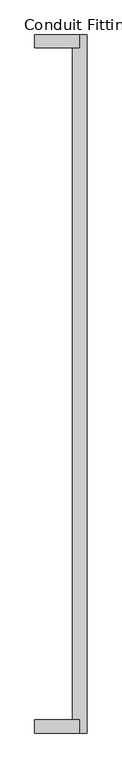
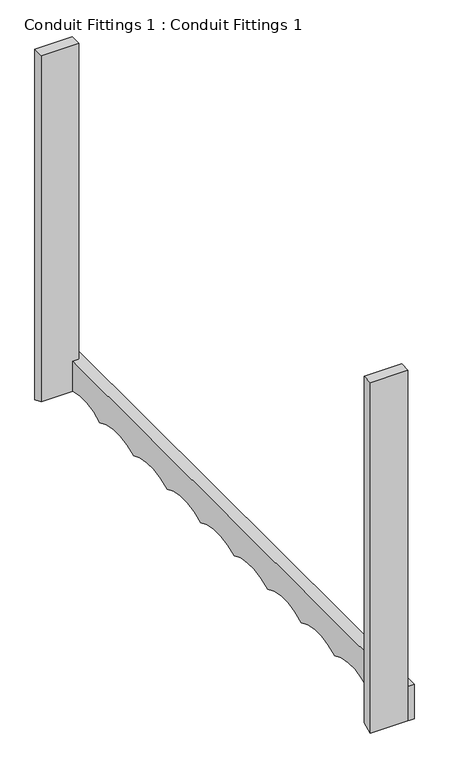
"""IFC4 building model written with IfcOpenShell, lengths in millimetres: cable carrier fitting geometry, Conduit Fittings 1 : Conduit Fittings 1."""

from ifc_helpers import new_model, si_unit, point, frame, frame_2d, origin, place, context, project, spatial, polyline, circle_curve, trimmed, segment, composite_curve, outline, extrude, source, transform, mapped, element, save


def conduit_fittings_1_conduit_fittings_1_9411e536(model_context):
    return source(origin(), model_context, "Body", "SweptSolid", [
        extrude(outline(composite_curve([segment(polyline([(3231.2168492, 10058.4), (3231.2168492, 2286.0)]), True, "CONTINUOUS"), segment(trimmed(circle_curve(frame_2d((2621.6168492, 1151.9587189)), 1287.5021504), [point((3231.2168492, 2286.0))], [point((3002.6168492, 2381.7964266))], True, "CARTESIAN"), True, "CONTINUOUS"), segment(polyline([(3002.6168492, 2381.7964266), (3002.6168492, 10058.4), (3231.2168492, 10058.4)]), True, "CONTINUOUS")], self_intersect=False)), frame((5842.9574466, 0.0, 0.0), z_axis=(1.0, 0.0, 0.0), x_axis=(0.0, 1.0, 0.0)), (0.0, 0.0, 1.0), 787.4),
        extrude(outline(composite_curve([segment(polyline([(-8732.1831508, 10058.4), (-8732.1831508, 2381.7964266)]), True, "CONTINUOUS"), segment(trimmed(circle_curve(frame_2d((-8351.1831508, 1151.9587189)), 1287.5021504), [point((-8732.1831508, 2381.7964266))], [point((-8960.7831508, 2286.0))], True, "CARTESIAN"), True, "CONTINUOUS"), segment(polyline([(-8960.7831508, 2286.0), (-8960.7831508, 10058.4), (-8732.1831508, 10058.4)]), True, "CONTINUOUS")], self_intersect=False)), frame((5842.9574466, 0.0, 0.0), z_axis=(1.0, 0.0, 0.0), x_axis=(0.0, 1.0, 0.0)), (0.0, 0.0, 1.0), 787.4),
        extrude(outline(composite_curve([segment(polyline([(3231.2168492, 3048.0), (3231.2168492, 2286.0)]), True, "CONTINUOUS"), segment(trimmed(circle_curve(frame_2d((2621.6168492, 1151.9587189)), 1287.5021504), [point((3231.2168492, 2286.0))], [point((2012.0168492, 2286.0))], True, "CARTESIAN"), True, "CONTINUOUS"), segment(trimmed(circle_curve(frame_2d((1402.4168492, 1151.9587189)), 1287.5021504), [point((2012.0168492, 2286.0))], [point((792.8168492, 2286.0))], True, "CARTESIAN"), True, "CONTINUOUS"), segment(trimmed(circle_curve(frame_2d((183.2168492, 1151.9587189)), 1287.5021504), [point((792.8168492, 2286.0))], [point((-426.3831508, 2286.0))], True, "CARTESIAN"), True, "CONTINUOUS"), segment(trimmed(circle_curve(frame_2d((-1035.9831508, 1151.9587189)), 1287.5021504), [point((-426.3831508, 2286.0))], [point((-1645.5831508, 2286.0))], True, "CARTESIAN"), True, "CONTINUOUS"), segment(trimmed(circle_curve(frame_2d((-2255.1831508, 1151.9587189)), 1287.5021504), [point((-1645.5831508, 2286.0))], [point((-2864.7831508, 2286.0))], True, "CARTESIAN"), True, "CONTINUOUS"), segment(trimmed(circle_curve(frame_2d((-3474.3831508, 1151.9587189)), 1287.5021504), [point((-2864.7831508, 2286.0))], [point((-4083.9831508, 2286.0))], True, "CARTESIAN"), True, "CONTINUOUS"), segment(trimmed(circle_curve(frame_2d((-4693.5831508, 1151.9587189)), 1287.5021504), [point((-4083.9831508, 2286.0))], [point((-5303.1831508, 2286.0))], True, "CARTESIAN"), True, "CONTINUOUS"), segment(trimmed(circle_curve(frame_2d((-5912.7831508, 1151.9587189)), 1287.5021504), [point((-5303.1831508, 2286.0))], [point((-6522.3831508, 2286.0))], True, "CARTESIAN"), True, "CONTINUOUS"), segment(trimmed(circle_curve(frame_2d((-7131.9831508, 1151.9587189)), 1287.5021504), [point((-6522.3831508, 2286.0))], [point((-7741.5831508, 2286.0))], True, "CARTESIAN"), True, "CONTINUOUS"), segment(trimmed(circle_curve(frame_2d((-8351.1831508, 1151.9587189)), 1287.5021504), [point((-7741.5831508, 2286.0))], [point((-8960.7831508, 2286.0))], True, "CARTESIAN"), True, "CONTINUOUS"), segment(polyline([(-8960.7831508, 2286.0), (-8960.7831508, 3048.0), (3231.2168492, 3048.0)]), True, "CONTINUOUS")], self_intersect=False)), frame((6504.2261671, 0.0, 0.0), z_axis=(1.0, 0.0, 0.0), x_axis=(0.0, 1.0, 0.0)), (0.0, 0.0, 1.0), 253.1312796),
    ])


if __name__ == "__main__":
    model = new_model("IFC4")
    model_context = context("Model", 3, world=origin())
    ifc_project = project(units=[si_unit("LENGTHUNIT", "METRE", prefix="MILLI")], contexts=[model_context])
    site = spatial("IfcSite", under=ifc_project)
    building = spatial("IfcBuilding", under=site)
    placement = place(None, origin())
    conduit_fittings_1_conduit_fittings_1_shape = conduit_fittings_1_conduit_fittings_1_9411e536(model_context)
    element("IfcCableCarrierFitting", 1, ObjectType="Conduit Fittings 1 : Conduit Fittings 1", at=placement, inside=building, context=model_context, shape_type="MappedRepresentation", body=[
        mapped(conduit_fittings_1_conduit_fittings_1_shape, transform((0.0, 0.0, 0.0), x_axis=(1.0, 0.0, 0.0), y_axis=(0.0, 1.0, 0.0), z_axis=(0.0, 0.0, 1.0))),
    ])
    save(model, "model.ifc")
